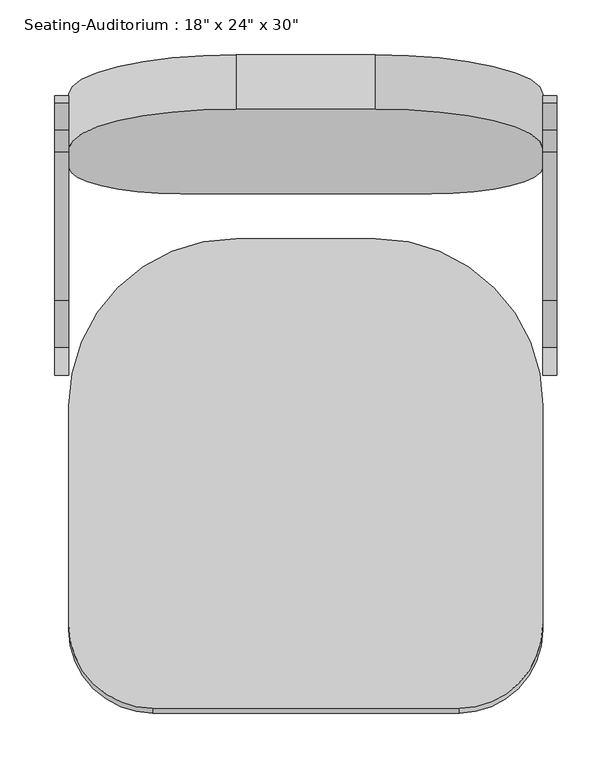
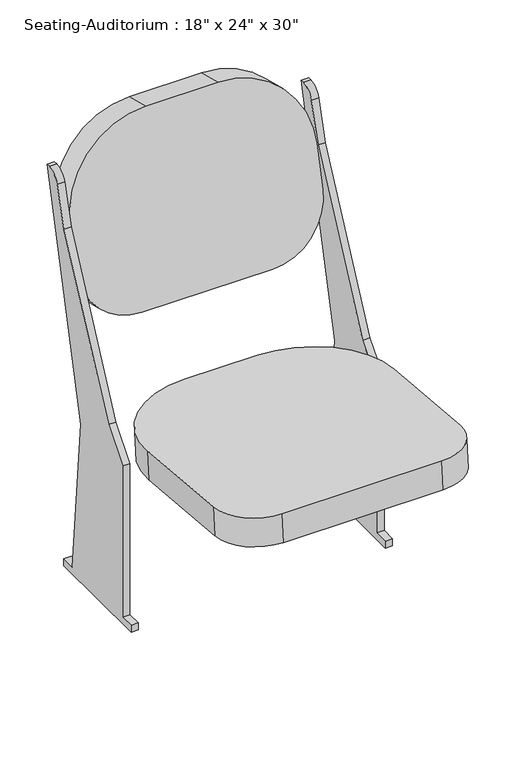
"""IFC4 building model written with IfcOpenShell, lengths in millimetres: furniture geometry."""

from ifc_helpers import new_model, si_unit, point, frame, frame_2d, origin, place, context, project, spatial, polyline, circle_curve, trimmed, segment, composite_curve, outline, extrude, source, transform, mapped, element, save


def furniture_2ec127df(model_context):
    return source(origin(), model_context, "Body", "SweptSolid", [
        extrude(outline(composite_curve([segment(trimmed(circle_curve(frame_2d((0.0, 152.4)), 152.4), [point((0.0, 0.0))], [point((-152.4, 152.4))], False, "CARTESIAN"), True, "CONTINUOUS"), segment(polyline([(-152.4, 152.4), (-152.4, 224.0588601)]), True, "CONTINUOUS"), segment(trimmed(circle_curve(frame_2d((-50.8, 224.0588601)), 101.6), [point((-152.4, 224.0588601))], [point((-50.8, 325.6588601))], False, "CARTESIAN"), True, "CONTINUOUS"), segment(polyline([(-50.8, 325.6588601), (177.8, 325.6588601)]), True, "CONTINUOUS"), segment(trimmed(circle_curve(frame_2d((177.8, 224.0588601)), 101.6), [point((177.8, 325.6588601))], [point((279.4, 224.0588601))], False, "CARTESIAN"), True, "CONTINUOUS"), segment(polyline([(279.4, 224.0588601), (279.4, 152.4)]), True, "CONTINUOUS"), segment(trimmed(circle_curve(frame_2d((127.0, 152.4)), 152.4), [point((279.4, 152.4))], [point((127.0, 0.0))], False, "CARTESIAN"), True, "CONTINUOUS"), segment(polyline([(127.0, 0.0), (0.0, 0.0)]), True, "CONTINUOUS")], self_intersect=False)), frame((224.2278689, 101.3396919, 755.9484479), z_axis=(0.0, -0.9717404775047361, 0.23605178325712217), x_axis=(-1.0, 0.0, 0.0)), (0.0, 0.0, 1.0), 50.8),
        extrude(outline(composite_curve([segment(polyline([(0.0, 0.0), (-279.4, 0.0)]), True, "CONTINUOUS"), segment(trimmed(circle_curve(frame_2d((-279.4, 76.2)), 76.2), [point((-279.4, 0.0))], [point((-355.6, 76.2))], False, "CARTESIAN"), True, "CONTINUOUS"), segment(polyline([(-355.6, 76.2), (-355.6, 276.4123505)]), True, "CONTINUOUS"), segment(trimmed(circle_curve(frame_2d((-203.2, 276.4123505)), 152.4), [point((-355.6, 276.4123505))], [point((-203.2, 428.8123506))], False, "CARTESIAN"), True, "CONTINUOUS"), segment(polyline([(-203.2, 428.8123506), (-76.2, 428.8123506)]), True, "CONTINUOUS"), segment(trimmed(circle_curve(frame_2d((-76.2, 276.4123505)), 152.4), [point((-76.2, 428.8123506))], [point((76.2, 276.4123505))], False, "CARTESIAN"), True, "CONTINUOUS"), segment(polyline([(76.2, 276.4123505), (76.2, 76.2)]), True, "CONTINUOUS"), segment(trimmed(circle_curve(frame_2d((0.0, 76.2)), 76.2), [point((76.2, 76.2))], [point((0.0, 0.0))], False, "CARTESIAN"), True, "CONTINUOUS")], self_intersect=False)), frame((300.4278689, -497.5245173, 321.2380213), z_axis=(0.0, 0.08715574274765496, 0.9961946980917459), x_axis=(1.0, 0.0, 0.0)), (0.0, 0.0, 1.0), 50.8),
        extrude(outline(composite_curve([segment(polyline([(13.3245902, 0.0), (-189.8754098, 0.0), (-189.8754098, 12.7), (-164.4754098, 12.7), (-164.4754098, 292.1), (-121.8491486, 342.9), (13.3245902, 622.3), (33.4611378, 692.7779166)]), True, "CONTINUOUS"), segment(trimmed(circle_curve(frame_2d((57.883846, 685.8)), 25.4), [point((33.4611378, 692.7779166))], [point((57.883846, 711.2))], False, "CARTESIAN"), True, "CONTINUOUS"), segment(polyline([(57.883846, 711.2), (64.1245902, 711.2), (-37.4754098, 292.1), (-12.0754098, 12.7), (13.3245902, 12.7), (13.3245902, 0.0)]), True, "CONTINUOUS")], self_intersect=False)), frame((-67.8721311, 0.0, 0.0), z_axis=(1.0, 0.0, 0.0), x_axis=(0.0, 1.0, 0.0)), (0.0, 0.0, 1.0), 12.7),
        extrude(outline(composite_curve([segment(polyline([(13.3245902, 12.7), (13.3245902, 0.0), (-189.8754098, 0.0), (-189.8754098, 12.7), (-164.4754098, 12.7), (-164.4754098, 292.1), (-121.8491486, 342.9), (13.3245902, 622.3), (33.4611378, 692.7779166)]), True, "CONTINUOUS"), segment(trimmed(circle_curve(frame_2d((57.883846, 685.8)), 25.4), [point((33.4611378, 692.7779166))], [point((57.883846, 711.2))], False, "CARTESIAN"), True, "CONTINUOUS"), segment(polyline([(57.883846, 711.2), (64.1245902, 711.2), (-37.4754098, 292.1), (-12.0754098, 12.7), (13.3245902, 12.7)]), True, "CONTINUOUS")], self_intersect=False)), frame((376.6278689, 0.0, 0.0), z_axis=(1.0, 0.0, 0.0), x_axis=(0.0, 1.0, 0.0)), (0.0, 0.0, 1.0), 12.7),
    ])


if __name__ == "__main__":
    model = new_model("IFC4")
    model_context = context("Model", 3, world=origin())
    ifc_project = project(units=[si_unit("LENGTHUNIT", "METRE", prefix="MILLI")], contexts=[model_context])
    site = spatial("IfcSite", under=ifc_project)
    building = spatial("IfcBuilding", under=site)
    placement = place(None, origin())
    furniture_shape = furniture_2ec127df(model_context)
    element("IfcFurniture", 1, ObjectType="Seating-Auditorium : 18\" x 24\" x 30\"", at=placement, inside=building, context=model_context, shape_type="MappedRepresentation", body=[
        mapped(furniture_shape, transform((0.0, 0.0, 0.0), x_axis=(1.0, 0.0, 0.0), y_axis=(0.0, 1.0, 0.0), z_axis=(0.0, 0.0, 1.0))),
    ])
    save(model, "model.ifc")

# Revit data of these elements
# Type "Seating-Auditorium : 18\" x 24\" x 30\""
#   Assembly Code = "E2020200"
#   Seat Material = Linen, Beige
#   Frame Material = Steel, Paint Finish, Dark Gray, Matte
#   Default Elevation = 0
# Element 1 (IfcFurniture, "Seating-Auditorium : 18\" x 24\" x 30\"")
#   Materials on its faces: "Steel, Paint Finish, Dark Gray, Matte", "Linen, Beige"
# Materials
#   "Linen, Beige": class "Textile", colour RGB 249 239 230, transparency 0, Description = "Linen, beige", Cost = 0
#   "Steel, Paint Finish, Dark Gray, Matte": class "Metal", colour RGB 0 0 0, transparency 0, Description = "Steel, paint finish, dark gray, matte", Cost = 0
